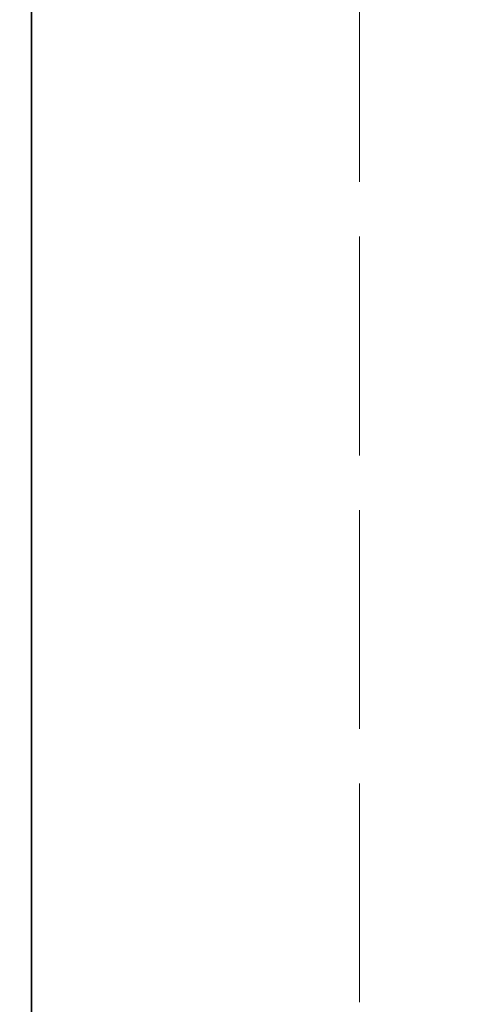
# Model space of a CAD drawing. Units: inches. Extents: x -1198 to -69, y -512 to 437.
# Tile 47 of 50: x -372 to -322, y 5 to 113. Entities that reach past the tile are written whole.
import ezdxf

# ---------------------------------------------------------------- set-up
doc = ezdxf.new("R2010")
doc.units = ezdxf.units.IN
doc.header["$MEASUREMENT"] = 0
doc.linetypes.add('ACAD_ISO02W100', pattern=[15, 12, -3])
for name, color, linetype, lineweight in [('A-ANNO-DIMS', 2, 'Continuous', 18), ('A-WALL', 7, 'Continuous', 35), ('C-PROP', 141, 'ACAD_ISO02W100', 18)]:
    doc.layers.add(name, color=color, linetype=linetype, lineweight=lineweight)
doc.styles.get("Standard").update_dxf_attribs({"font": 'arial.ttf'})
doc.dimstyles.get("Standard").update_dxf_attribs({"dimtxt": 6, "dimasz": 6, "dimexe": 0.18, "dimexo": 0.0625, "dimgap": 0.09, "dimtad": 0, "dimtih": 1, "dimtoh": 1, "dimdec": 0, "dimzin": 0, "dimdsep": 46, "dimlunit": 4, "dimtxsty": 'Standard', "dimblk": 'OBLIQUE', "dimcen": 0.09, "dimadec": 0, "dimazin": 0, "dimtfac": 1, "dimtdec": 0, "dimtofl": 0, "dimtmove": 0, "dimatfit": 3, "dimfxl": 1, "dimtolj": 1, "dimtzin": 0, "dimarcsym": 0})

# ---------------------------------------------------------------- blocks, each defined once
blk = doc.blocks.new('_Oblique')
at = {"color": 0, "linetype": 'ByBlock', "lineweight": -2}
blk.add_line((-0.5, -0.5), (0.5, 0.5), dxfattribs=at)
blk = doc.blocks.new('*D63')
at = {"layer": 'A-ANNO-DIMS', "color": 0, "lineweight": -2, "ltscale": 10, "transparency": 16777216}
for p, q in [((-370.69, 263.23), (-79.37, 263.23)), ((-79.55, 263.23), (-79.55, 20.38)), ((-79.55, -228.77), (-79.55, 14.07)), ((-370.69, -228.77), (-79.37, -228.77))]:
    blk.add_line(p, q, dxfattribs=at)
at = {"layer": 'DEFPOINTS', "color": 0, "ltscale": 10, "transparency": 16777216}
for p in [(-370.75, 263.23), (-79.55, 263.23), (-370.75, -228.77)]:
    blk.add_point(p, dxfattribs=at)
at = {"layer": 'A-ANNO-DIMS', "color": 0, "lineweight": -2, "ltscale": 10, "transparency": 16777216, "xscale": 6, "yscale": 6, "zscale": 6}
for p, rotation in [((-79.55, 263.23), 90), ((-79.55, -228.77), 270)]:
    blk.add_blockref('_Oblique', p, dxfattribs=dict(at, rotation=rotation))
at = {"layer": 'A-ANNO-DIMS', "color": 0, "ltscale": 10, "transparency": 16777216, "insert": (-79.55, 17.23), "char_height": 6, "attachment_point": 5}
blk.add_mtext('\\A1;492', dxfattribs=at)

msp = doc.modelspace()

# ---------------------------------------------------------------- linework, layer by layer
at = {"layer": 'A-WALL', "ltscale": 10}
msp.add_line((-370.7509, -228.7723), (-370.7509, 263.2277), dxfattribs=at)
at = {"layer": 'C-PROP', "ltscale": 2}
msp.add_lwpolyline([(-1054.7509, 299.2277), (-334.7509, 299.2277), (-334.7509, -264.7723), (-1054.7509, -264.7723)], close=True, dxfattribs=at)

# ---------------------------------------------------------------- dimensions: what is measured, and where the dimension line sits
at = {"layer": 'A-ANNO-DIMS', "ltscale": 10}
dim = msp.add_linear_dim(base=(-79.5507, 263.2277), p1=(-370.7509, -228.7723), p2=(-370.7509, 263.2277), angle=90, dimstyle='Standard', override={"dimdec": 0, "dimlfac": 1, "dimrnd": 0, "dimzin": 0, "dimdsep": 46, "dimlunit": 2}, dxfattribs=at)
dim.commit()
dim.dimension.update_dxf_attribs({"geometry": '*D63', "text_midpoint": (-79.5507, 17.2277)})

doc.saveas('drawing.dxf')
